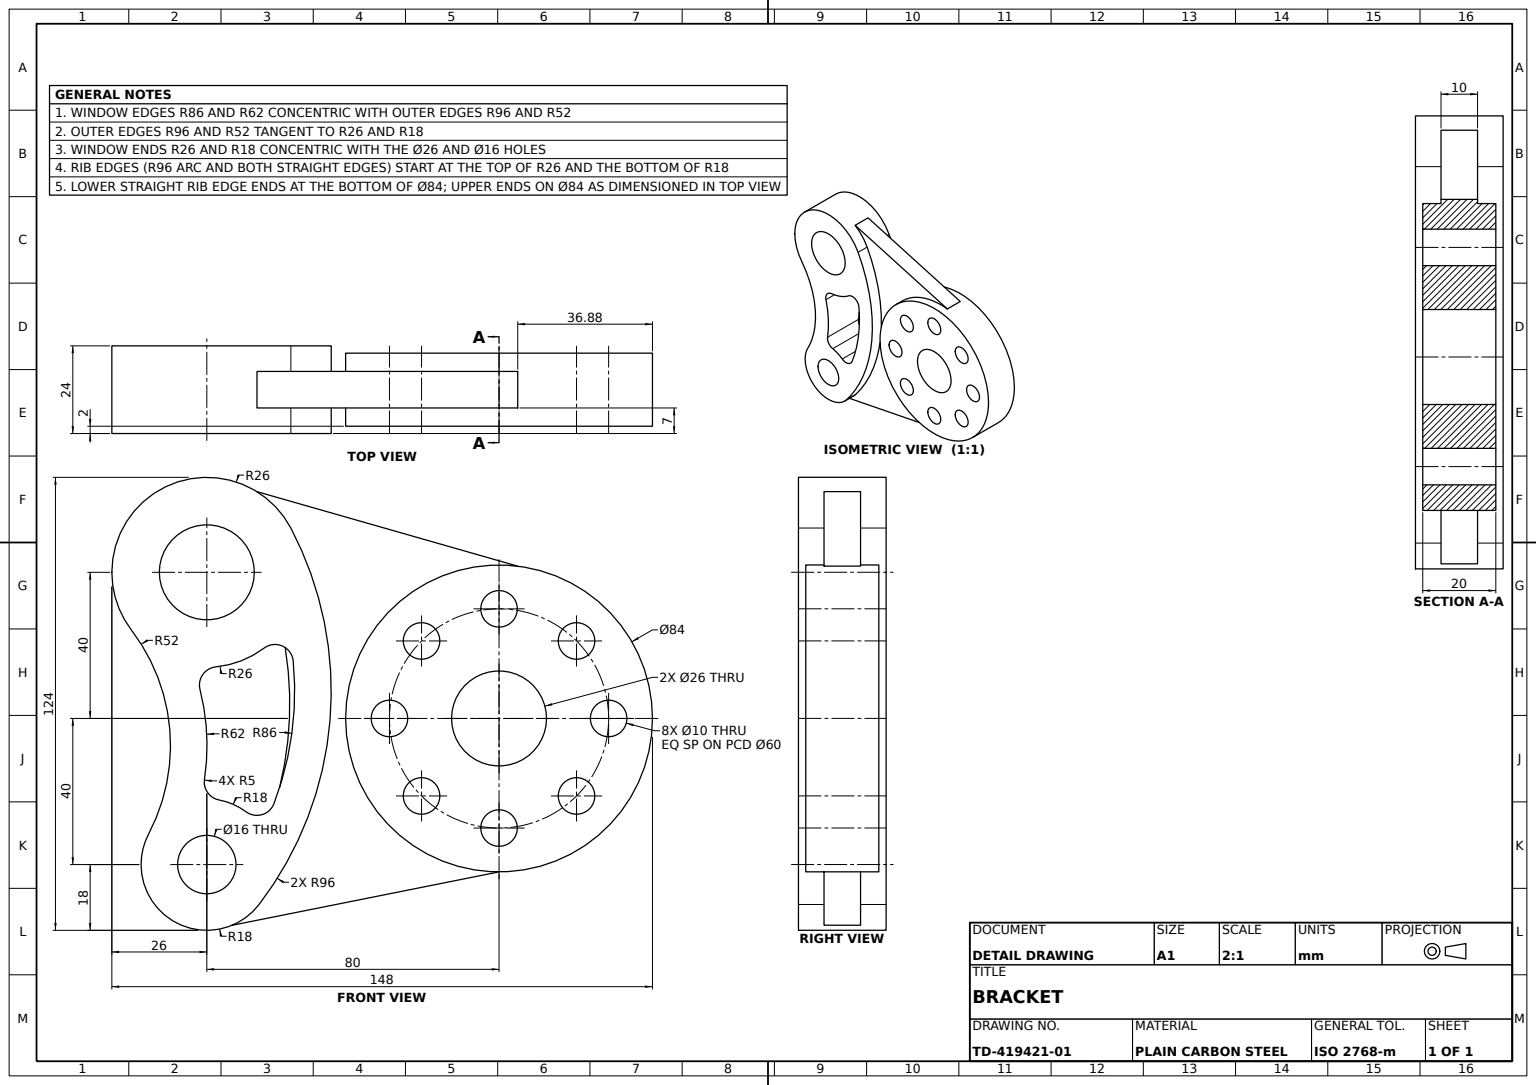
SolidWorks part; units mm, degrees
material "Plain Carbon Steel"
ref_plane "Front Plane" through (0, 0, 0) normal (0, 0, 1) x (1, 0, 0)
ref_plane "Top Plane" through (0, 0, 0) normal (0, 1, 0) x (1, 0, 0)
ref_plane "Right Plane" through (0, 0, 0) normal (1, 0, 0) x (0, 0, -1)
sketch "Link Plate Profile" plane through (0, 0, 0) normal (0, 0, 1) x (1, 0, 0)
  line L0 (0, 0) -> (-80, 0) construction
  line L1 (-80, 0) -> (-80, -40) construction
  line L2 (-80, 0) -> (-80, 40) construction
  circle A0 centre (0, 0) radius 42
  arc A1 (-80, 14) -> (-64.3389, 19.2459) centre (-80, 40) ccw
  circle A2 centre (-80, 40) radius 13
  arc A3 (-69.2699, -25.5479) -> (-80, -22) centre (-80, -40) ccw
  circle A4 centre (-80, -40) radius 8
  arc A5 (-56.9917, 52.1086) -> (-65.7049, -50.9385) centre (-141.9455, 7.4) cw
  arc A6 (-100.6485, 24.2) -> (-95.9288, -31.6171) centre (-141.9455, -7.4) cw
  arc A7 (-56.3508, 15.7396) -> (-61.6191, -23.3194) centre (-141.9455, 7.4) cw
  arc A8 (-81.8652, 7.909) -> (-80.6408, -16.6594) centre (-141.9455, -7.4) cw
  arc A9 (-65.841, 47.4514) -> (-73.6466, -44.8615) centre (-141.9455, 7.4) cw construction
  arc A10 (-92.7068, 30.2769) -> (-87.0795, -36.2743) centre (-141.9455, -7.4) cw construction
  arc A11 (-56.3508, 15.7396) -> (-64.3389, 19.2459) centre (-61.3272, 15.2548) ccw
  arc A12 (-77.5007, 14.1204) -> (-81.8652, 7.909) centre (-77.02, 9.1436) ccw
  arc A13 (-56.9917, 52.1086) -> (-100.6485, 24.2) centre (-80, 40) ccw
  arc A14 (-80.6408, -16.6594) -> (-76.6323, -22.3178) centre (-75.6969, -17.4061) ccw
  arc A15 (-69.2699, -25.5479) -> (-61.6191, -23.3194) centre (-66.2893, -21.5334) ccw
  arc A16 (-95.9288, -31.6171) -> (-65.7049, -50.9385) centre (-80, -40) ccw
  dimension "D1" = 84
  dimension "D2" = 52
  dimension "D3" = 26
  dimension "D4" = 36
  dimension "D5" = 16
  dimension "D9" = 96
  dimension "D10" = 52
  dimension "D13" = 10
  dimension "D14" = 10
  dimension "D15" = 10
  dimension "D16" = 10
  dimension "D6" = 80
  dimension "D7" = 40
  dimension "D8" = 40
  dimension "D11" = 10
  dimension "D12" = 10
extrude "Link Plate" add sketch "Link Plate Profile" along normal blind 24
ref_plane "Hub Offset Plane" through (0, 0, 12) normal (0, 0, 1) x (1, 0, 0)
sketch "Hub Disc Profile Ø84" plane through (0, 0, 12) normal (0, 0, 1) x (1, 0, 0)
  circle A0 centre (0, 0) radius 42
  dimension "D1" = 84
extrude "Hub Disc Ø84" add sketch "Hub Disc Profile Ø84" along normal mid plane 20 separate body
sketch "Rib Profile" plane through (0, 0, 12) normal (0, 0, 1) x (1, 0, 0)
  line L0 (-80, 66) -> (5.1163, 41.6872)
  line L1 (0, -42) -> (-80, -58)
  arc A0 (-56.9917, 52.1086) -> (-100.6485, 24.2) centre (-80, 40) ccw construction
  circle A1 centre (0, 0) radius 42 construction
  arc A2 (-95.9288, -31.6171) -> (-65.7049, -50.9385) centre (-80, -40) ccw construction
  arc A3 (5.1163, 41.6872) -> (0, -42) centre (0, 0) ccw
  arc A4 (-80, 66) -> (-80, -58) centre (-153.2939, 4) cw
  dimension "D1" = 96
  dimension "D2" = 73.2939
  dimension "D3" = 158.4103
extrude "Hub Rib" add sketch "Rib Profile" along normal mid plane 10
sketch "Hub Centre Bore Sketch" plane through (0, 0, 22) normal (0, 0, 1) x (1, 0, 0)
  circle A0 centre (0, 0) radius 13
  dimension "D1" = 26
extrude "Hub Centre Bore" cut sketch "Hub Centre Bore Sketch" against normal through all
sketch "Hub Hole Sketch" plane through (0, 0, 22) normal (0, 0, 1) x (1, 0, 0)
  line L0 (0, 0) -> (0, 30) construction
  circle A0 centre (0, 30) radius 5
  circle A1 centre (0, 0) radius 13 construction
  dimension "D1" = 10
  dimension "D2" = 30
extrude "Hub Hole" cut sketch "Hub Hole Sketch" against normal through all
pattern_circular "Hub Hole Pattern 8x" count 8 over 360 about axis through (0, 0, 0) along (0, 0, 1) of "Hub Hole"
